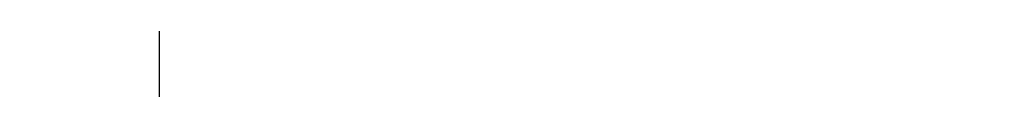
# Model space of a CAD drawing. Units: inches. Extents: x 2091 to 2899, y 967 to 2217.
# Tile 11 of 256: x 2312 to 2351, y 1088 to 1090. Entities that reach past the tile are written whole.
import ezdxf

# ---------------------------------------------------------------- set-up
doc = ezdxf.new("R2010")
doc.units = ezdxf.units.IN
doc.layers.add('A-ANNO-DIMS', color=2, linetype='Continuous', lineweight=18)
doc.styles.get("Standard").update_dxf_attribs({"font": 'arial.ttf'})
doc.dimstyles.new('ISO-25', dxfattribs={"dimtxt": 4, "dimasz": 4, "dimexe": 1.25, "dimexo": 0.625, "dimtad": 1, "dimdec": 0, "dimlunit": 3, "dimtxsty": 'Standard', "dimcen": 2.5, "dimadec": 0, "dimazin": 0, "dimtfac": 1, "dimtdec": 0, "dimtmove": 0, "dimatfit": 3, "dimfxl": 1, "dimarcsym": 0})

# ---------------------------------------------------------------- blocks, each defined once
blk = doc.blocks.new('*D68')
at = {"layer": 'A-ANNO-DIMS', "color": 0, "lineweight": -2, "transparency": 16777216}
for p, q in [((2317.144, 1535.794), (2317.144, 969.464)), ((2459.384, 1535.794), (2459.384, 969.464)), ((2321.144, 970.714), (2455.384, 970.714))]:
    blk.add_line(p, q, dxfattribs=at)
at = {"layer": 'A-ANNO-DIMS', "color": 0, "transparency": 16777216}
for points in [[(2321.144, 971.381), (2321.144, 970.048), (2317.144, 970.714)], [(2455.384, 971.381), (2455.384, 970.048), (2459.384, 970.714)]]:
    blk.add_solid(points, dxfattribs=at)
at = {"layer": 'Defpoints', "color": 0, "transparency": 16777216}
for p in [(2317.144, 1536.419), (2459.384, 1536.419), (2459.384, 970.714)]:
    blk.add_point(p, dxfattribs=at)
at = {"layer": 'A-ANNO-DIMS', "color": 0, "transparency": 16777216, "insert": (2388.264, 973.382), "char_height": 4, "attachment_point": 5}
blk.add_mtext('11\'-10"', dxfattribs=at)
blk = doc.blocks.new('*D71')
at = {"layer": 'A-ANNO-DIMS', "color": 0, "lineweight": -2, "transparency": 16777216}
for p, q in [((2212.144, 1351.294), (2212.144, 969.464)), ((2452.144, 1351.294), (2452.144, 969.464)), ((2216.144, 970.714), (2448.144, 970.714))]:
    blk.add_line(p, q, dxfattribs=at)
at = {"layer": 'A-ANNO-DIMS', "color": 0, "transparency": 16777216}
for points in [[(2216.144, 971.381), (2216.144, 970.048), (2212.144, 970.714)], [(2448.144, 971.381), (2448.144, 970.048), (2452.144, 970.714)]]:
    blk.add_solid(points, dxfattribs=at)
at = {"layer": 'Defpoints', "color": 0, "transparency": 16777216}
for p in [(2212.144, 1351.919), (2452.144, 1351.919), (2452.144, 970.714)]:
    blk.add_point(p, dxfattribs=at)
at = {"layer": 'A-ANNO-DIMS', "color": 0, "transparency": 16777216, "insert": (2332.144, 973.382), "char_height": 4, "attachment_point": 5}
blk.add_mtext('20\'-0"', dxfattribs=at)

msp = doc.modelspace()

# ---------------------------------------------------------------- dimensions: what is measured, and where the dimension line sits
at = {"layer": 'A-ANNO-DIMS'}
for base, p1, p2, picture, middle in [((2459.384, 970.714), (2317.144, 1536.419), (2459.384, 1536.419), '*D68', (2388.264, 973.382)), ((2452.144, 970.714), (2212.144, 1351.919), (2452.144, 1351.919), '*D71', (2332.144, 973.382))]:
    dim = msp.add_linear_dim(base=base, p1=p1, p2=p2, dimstyle='ISO-25', override={"dimdec": 1, "dimlfac": 1, "dimrnd": 0, "dimzin": 1, "dimdsep": 46, "dimlunit": 4, "dimfrac": 2}, dxfattribs=at)
    dim.commit()
    dim.dimension.update_dxf_attribs({"geometry": picture, "text_midpoint": middle})

doc.saveas('drawing.dxf')
